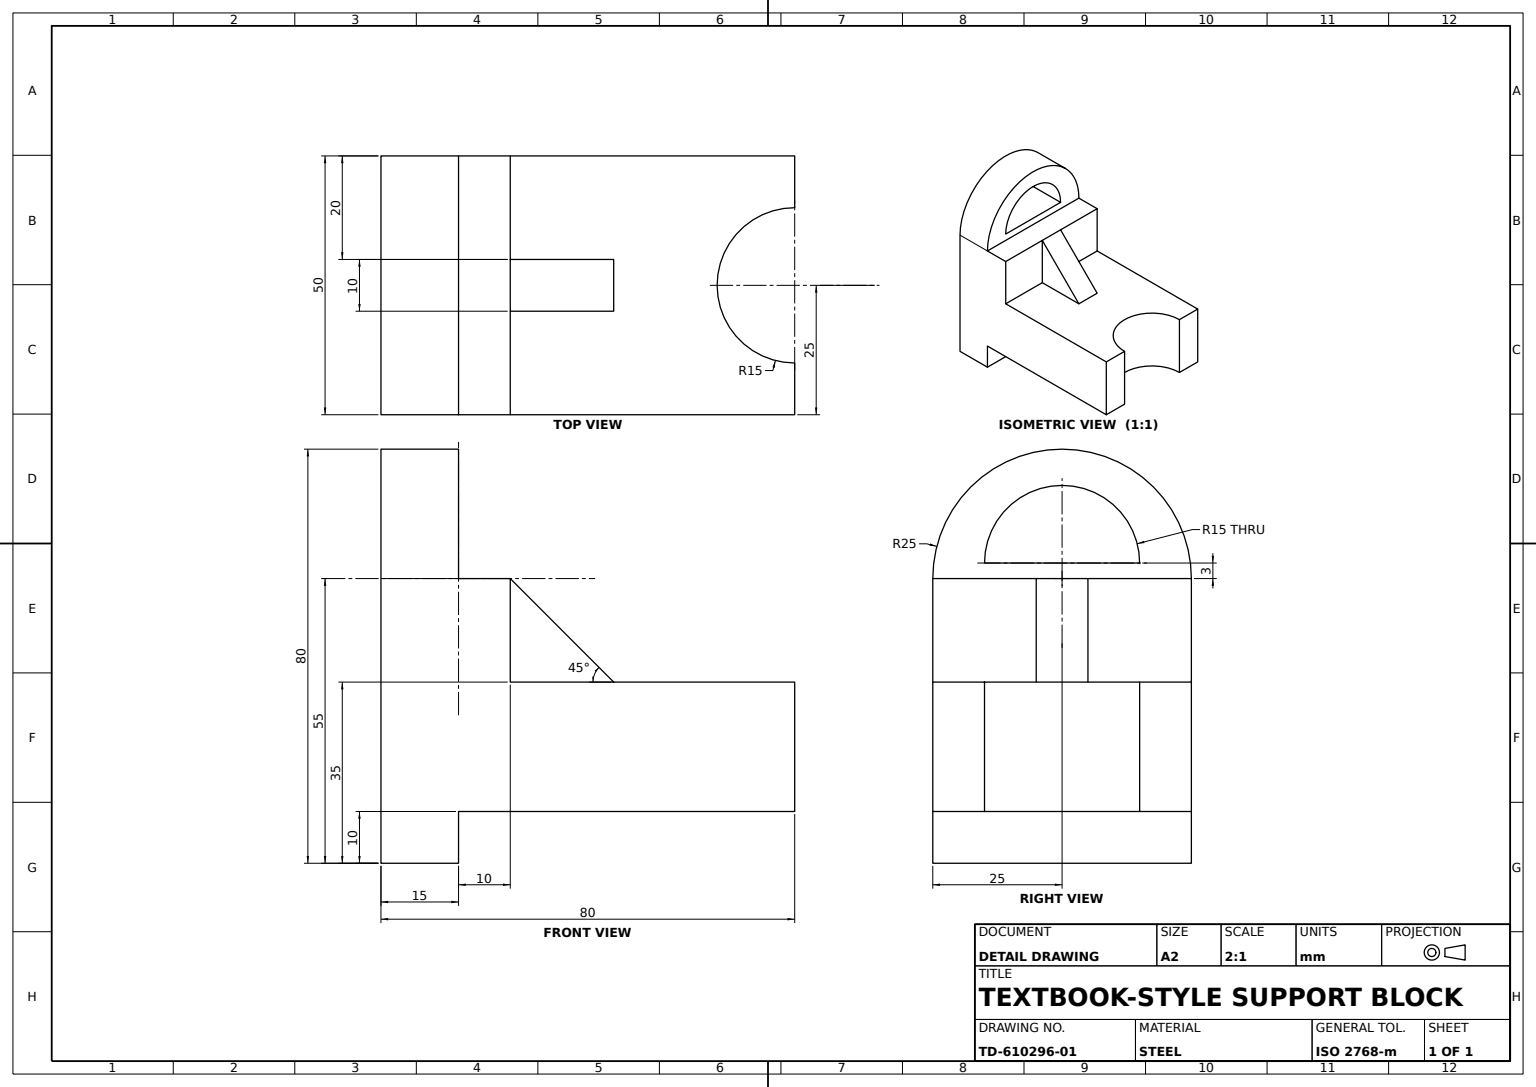
from build123d import *

# Parameters (mm, degrees)
BASE_BLOCK_50MM_DEPTH         = 50
STEP_BOSS_SKETCH_W            = 50
STEP_BOSS_SKETCH_H            = 55
STEP_BOSS_10MM_DEPTH          = 10
STEP_CUT_SKETCH_W             = 50
STEP_CUT_SKETCH_H             = 55
STEP_CUT_10MM_DEPTH           = 10
UPRIGHT_PAD_SKETCH_W          = 50
UPRIGHT_PAD_SKETCH_H          = 55
UPRIGHT_PAD_5MM_DEPTH         = 5
ARCH_BOSS_15MM_DEPTH          = 15
UPPER_BLOCK_SKETCH_W          = 50
UPPER_BLOCK_SKETCH_H          = 20
UPPER_BLOCK_10MM_DEPTH        = 10
BASE_SEMICIRCULAR_NOTCH_DEPTH = 15
ARCH_SEMICIRCULAR_CUT_DEPTH   = 25
SUPPORT_RIB_30MM_DEPTH        = 30
RIB_TRIM_CUT_20MM_DEPTH       = 20


with BuildPart() as part:
    # Base Profile Sketch → Base Block 50mm (new body)
    with BuildSketch(Plane.XY):
        Polygon((0, 0), (0, 55), (10, 55), (10, 35), (75, 35), (75, 10), (10, 10), (10, 0), align=None)
    extrude(amount=BASE_BLOCK_50MM_DEPTH)

    # Step Boss Sketch → Step Boss 10mm (add)
    with BuildSketch(Plane.ZY):
        with Locations((25, 27.5)):
            Rectangle(STEP_BOSS_SKETCH_W, STEP_BOSS_SKETCH_H)
    extrude(amount=STEP_BOSS_10MM_DEPTH)

    # Step Cut Sketch → Step Cut 10mm (cut)
    with BuildSketch(Plane.ZY.offset(10)):
        with Locations((25, 27.5)):
            Rectangle(STEP_CUT_SKETCH_W, STEP_CUT_SKETCH_H)
    extrude(amount=-STEP_CUT_10MM_DEPTH, mode=Mode.SUBTRACT)

    # Upright Pad Sketch → Upright Pad 5mm (add)
    with BuildSketch(Plane.ZY):
        with Locations((25, 27.5)):
            Rectangle(UPRIGHT_PAD_SKETCH_W, UPRIGHT_PAD_SKETCH_H)
    extrude(amount=UPRIGHT_PAD_5MM_DEPTH)

    # Arch Boss Sketch R25 → Arch Boss 15mm (add)
    with BuildSketch(Plane.ZY.offset(5)):
        with BuildLine():
            Line((0, 55), (50, 55))
            ThreePointArc((50, 55), (25, 80), (0, 55))
        make_face()
    extrude(amount=-ARCH_BOSS_15MM_DEPTH)

    # Upper Block Sketch → Upper Block 10mm (add)
    with BuildSketch(Plane(origin=(10, 0, 0), x_dir=(0, 0, -1), z_dir=(1, 0, 0))):
        with Locations((-25, 45)):
            Rectangle(UPPER_BLOCK_SKETCH_W, UPPER_BLOCK_SKETCH_H)
    extrude(amount=UPPER_BLOCK_10MM_DEPTH)

    # Base Notch Sketch Ø30 → Base Semicircular Notch (cut)
    with BuildSketch(Plane(origin=(10, 0, 0), x_dir=(0, 0, -1), z_dir=(1, 0, 0))):
        with BuildLine():
            Line((-40, 58), (-25, 58))
            Line((-25, 58), (-10, 58))
            ThreePointArc((-10, 58), (-25, 73), (-40, 58))
        make_face()
    extrude(amount=-BASE_SEMICIRCULAR_NOTCH_DEPTH, mode=Mode.SUBTRACT)

    # Arch Cut Sketch Ø30 → Arch Semicircular Cut (cut)
    with BuildSketch(Plane(origin=(0, 35, 0), x_dir=(1, 0, 0), z_dir=(0, 1, 0))):
        with BuildLine():
            Line((75, -10), (75, -40))
            ThreePointArc((75, -40), (60, -25), (75, -10))
        make_face()
    extrude(amount=-ARCH_SEMICIRCULAR_CUT_DEPTH, mode=Mode.SUBTRACT)

    # Rib Sketch → Support Rib 30mm (add)
    with BuildSketch(Plane.XY.offset(50)):
        Polygon((20, 55), (20, 35), (40, 35), align=None)
    extrude(amount=-SUPPORT_RIB_30MM_DEPTH)

    # Rib Trim Sketch → Rib Trim Cut 20mm (cut)
    with BuildSketch(Plane.XY.offset(50)):
        Polygon((20, 55), (20, 35), (40, 35), align=None)
    extrude(amount=-RIB_TRIM_CUT_20MM_DEPTH, mode=Mode.SUBTRACT)


solid = part.part
